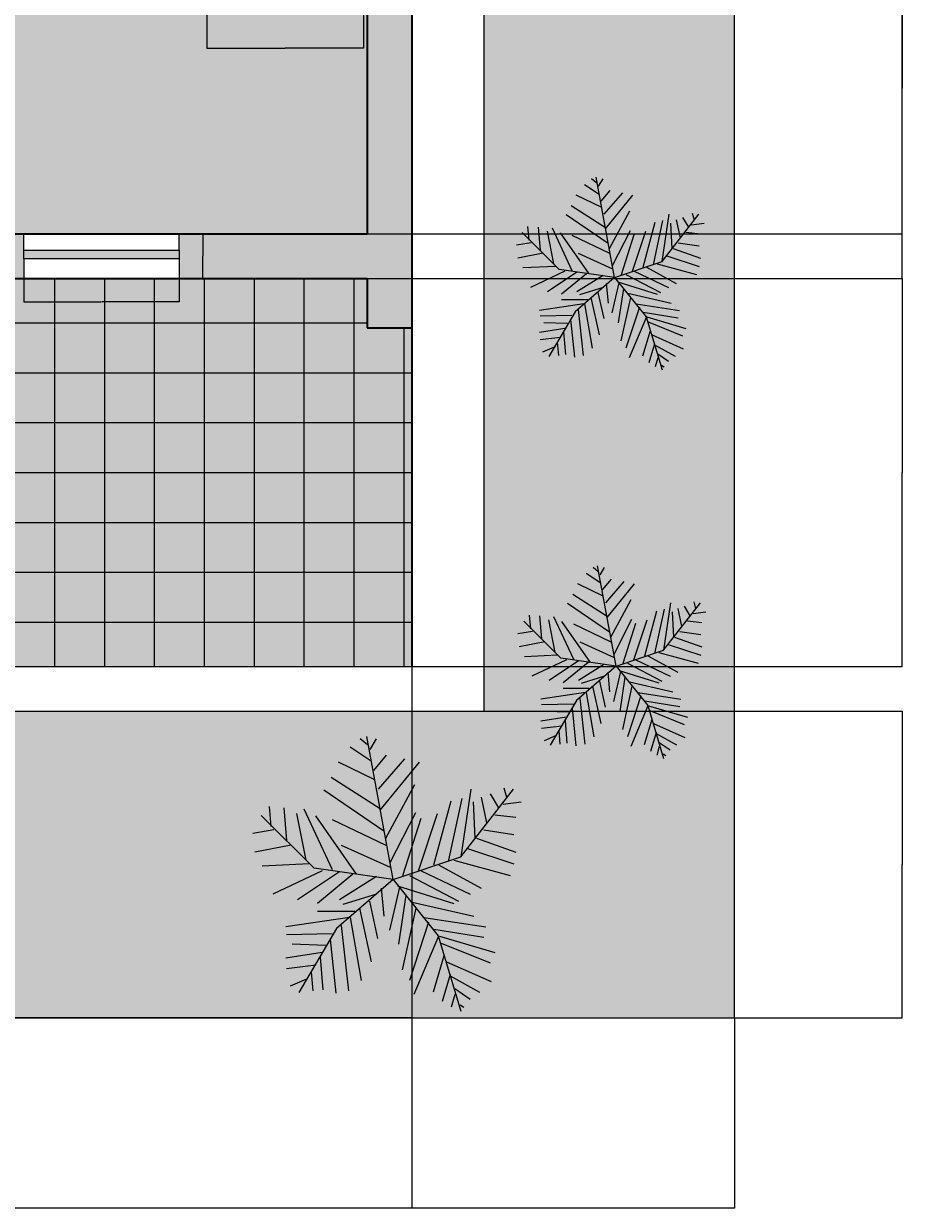
# Model space of a CAD drawing. Units: millimetres. Extents: x -229 to 16545, y -10488 to 4272.
# Tile 8 of 29: x 12015 to 16545, y -10230 to -4126. Entities that reach past the tile are written whole.
import ezdxf

# ---------------------------------------------------------------- set-up
doc = ezdxf.new("R2010")
doc.units = ezdxf.units.MM
for name, color, linetype, lineweight in [('A-ANNO-DIMS', 2, 'Continuous', 18), ('A-GLAZ', 4, 'Continuous', 18), ('A-WALL', 7, 'Continuous', 35), ('L-PLNT-BEDS', 82, 'Continuous', 18), ('L-PLNT-TREE', 80, 'Continuous', 18), ('L-PVMT', 7, 'Continuous', 18), ('L-PVMT-JNTS', 8, 'Continuous', 13)]:
    doc.layers.add(name, color=color, linetype=linetype, lineweight=lineweight)
for name, color, linetype, lineweight, true_color in [('A-FLOR-PATT', 254, 'Continuous', 13, 0xfeeab9), ('A-WALL-PATT', 18, 'Continuous', 13, 0x000000), ('L-PLNT-PATT', 116, 'Continuous', 13, 0x136734), ('L-PVMT-PATT', 252, 'Continuous', 13, 0x939598)]:
    doc.layers.add(name, color=color, linetype=linetype, lineweight=lineweight, true_color=true_color)
doc.styles.get("Standard").update_dxf_attribs({"font": 'arial.ttf'})
doc.dimstyles.get("Standard").update_dxf_attribs({"dimtxt": 0.18, "dimasz": 0.18, "dimexe": 0.18, "dimexo": 0.0625, "dimgap": 0.09, "dimtad": 0, "dimtih": 1, "dimtoh": 1, "dimdec": 4, "dimzin": 0, "dimdsep": 46, "dimtxsty": 'Standard', "dimcen": 0.09, "dimadec": 0, "dimazin": 0, "dimtfac": 1, "dimtdec": 4, "dimtofl": 0, "dimtmove": 0, "dimatfit": 3, "dimfxl": 1, "dimtolj": 1, "dimtzin": 0, "dimarcsym": 0})

# ---------------------------------------------------------------- blocks, each defined once
blk = doc.blocks.new('*U18')
for p, q in [((0, 0), (-10.5, 57)), ((-8.737, 47.138), (-17.069, 52.711)), ((-10.186, 53.64), (-13.084, 55.962)), ((-9.099, 51.782), (-6.563, 55.962)), ((-7.65, 43.423), (-2.578, 49.46)), ((-5.839, 35.992), (4.667, 48.067)), ((-7.288, 39.707), (-21.778, 46.673)), ((-5.114, 27.632), (10.463, 46.673)), ((-5.114, 28.097), (-24.676, 40.636)), ((-2.941, 16.486), (8.652, 37.85)), ((-3.665, 19.273), (-27.574, 35.527)), ((27, 9), (48, 36)), ((27.127, 9.056), (31.112, 35.992)), ((38.719, 34.134), (41.979, 28.561)), ((44.153, 36.456), (45.239, 32.741)), ((-48.585, 21.131), (-49.309, 29.026)), ((-43.513, 28.561), (-42.427, 15.558)), ((16.259, 5.805), (23.142, 31.348)), ((22.055, 7.198), (27.489, 32.277)), ((31.836, 30.883), (32.561, 16.486)), ((35.096, 32.741), (37.27, 22.524)), ((43.791, 29.954), (51.036, 30.883)), ((-31.5, 4.5), (-52.5, 25.5)), ((-38.442, 26.239), (-34.819, 7.663)), ((-35.544, 28.097), (-24.314, 3.947)), ((-14.533, 2.09), (-30.834, 25.31)), ((-24.314, 23.917), (-2.941, 13.7)), ((-1.129, 6.734), (9.014, 26.704)), ((3.942, 1.625), (11.187, 24.381)), ((10.101, 3.483), (17.708, 26.239)), ((40.53, 25.775), (48.862, 24.846)), ((-47.498, 19.737), (-55.83, 18.344)), ((36.183, 19.737), (48.137, 17.88)), ((33.285, 16.486), (48.862, 10.913)), ((-40.615, 13.7), (-55.105, 10.913)), ((-20.691, 13.7), (-1.129, 4.876)), ((29.662, 12.307), (48.137, 6.269)), ((-33.37, 6.269), (-52.207, 5.34)), ((0, 0), (27, 9)), ((18.07, 5.805), (35.096, -3.483)), ((24.229, 7.663), (46.688, 1.625)), ((-28.299, 3.483), (-47.86, -5.805)), ((-21.416, 3.018), (-38.079, -8.128)), ((0, 0), (-31.5, 4.5)), ((-15.982, 2.09), (-30.11, -9.521)), ((0, 0), (-22.5, -19.5)), ((-6.563, 1.161), (-21.416, -8.128)), ((0, 0), (18, -22.5)), ((6.478, 1.625), (26.04, -8.592)), ((11.187, 3.483), (30.749, -5.805)), ((-4.752, -3.483), (-3.665, -14.629)), ((2.493, -3.019), (-1.491, -20.202)), ((1.769, -2.555), (24.229, -9.521)), ((-6.563, -5.805), (-19.967, -9.985)), ((-9.461, -8.592), (-6.201, -23.453)), ((5.029, -6.27), (2.131, -25.775)), ((7.565, -9.056), (32.198, -14.629)), ((-15.257, -12.772), (-30.11, -12.772)), ((-13.446, -11.378), (-8.737, -32.741)), ((9.014, -11.378), (3.58, -35.992)), ((-17.431, -15.094), (-42.789, -18.809)), ((-20.691, -18.345), (-17.793, -44.352)), ((-17.069, -15.094), (-12.721, -40.172)), ((14.085, -16.951), (6.478, -40.172)), ((12.274, -15.094), (36.907, -18.809)), ((-24.314, -21.596), (-42.427, -22.06)), ((-22.5, -19.5), (-37.5, -45)), ((18.07, -22.524), (8.289, -45.745)), ((16.259, -19.738), (36.183, -22.989)), ((18, -22.5), (27, -52.5)), ((18.433, -22.524), (40.53, -29.026)), ((-26.849, -26.24), (-40.253, -25.775)), ((-25.038, -23.918), (-22.865, -45.281)), ((19.157, -25.311), (38.719, -33.206)), ((-28.299, -29.026), (-42.789, -31.348)), ((-29.023, -30.884), (-27.936, -43.887)), ((20.244, -30.419), (15.897, -44.816)), ((21.331, -32.741), (39.081, -40.636)), ((-30.834, -34.135), (-42.427, -35.528)), ((-32.646, -36.921), (-31.921, -44.352)), ((-34.457, -39.708), (-40.978, -42.494)), ((22.78, -37.85), (19.519, -48.532)), ((22.78, -38.314), (34.372, -44.816)), ((24.591, -45.745), (23.142, -50.854)), ((24.591, -43.423), (30.749, -47.603)), ((26.764, -49.925), (28.213, -50.854))]:
    blk.add_line(p, q)
blk = doc.blocks.new('WIN-802')
at = {"transparency": 33554687}
for p, q in [((0, 145), (0, 230)), ((802.3, 145), (802.3, 230)), ((0, 100.7), (0, 0)), ((802.3, 100.7), (802.3, 0))]:
    blk.add_line(p, q, dxfattribs=at)
blk.add_lwpolyline([(0, 145), (802.3, 145), (802.3, 100.7), (0, 100.7)], close=True, dxfattribs=at)
blk = doc.blocks.new('*D25')
at = {"layer": 'A-ANNO-DIMS', "color": 0, "lineweight": -2, "transparency": 16777216}
for p, q in [((12015.2, -5438.3), (12015.2, -5558.8)), ((12817.5, -5438.3), (12817.5, -5558.8)), ((12015.3, -5558.6), (12415.2, -5558.6)), ((12817.3, -5558.6), (12417.5, -5558.6))]:
    blk.add_line(p, q, dxfattribs=at)
at = {"layer": 'A-ANNO-DIMS', "color": 0, "transparency": 16777216}
for points in [[(12015.3, -5558.6), (12015.3, -5558.7), (12015.2, -5558.6)], [(12817.3, -5558.6), (12817.3, -5558.7), (12817.5, -5558.6)]]:
    blk.add_solid(points, dxfattribs=at)
at = {"layer": 'Defpoints', "color": 0, "transparency": 16777216}
for p in [(12015.2, -5438.3), (12817.5, -5438.3), (12817.5, -5558.6)]:
    blk.add_point(p, dxfattribs=at)
at = {"layer": 'A-ANNO-DIMS', "color": 0, "transparency": 16777216, "insert": (12416.3, -5558.6), "char_height": 0.18, "attachment_point": 5}
blk.add_mtext('\\A1;WINDOW 802 TYP.', dxfattribs=at)
blk = doc.blocks.new('*D26')
at = {"layer": 'A-ANNO-DIMS', "color": 0, "lineweight": -2, "transparency": 16777216}
for p, q in [((12817.6, -5208.3), (12938, -5208.3)), ((12937.9, -5208.5), (12937.9, -5323.1)), ((12937.9, -5438.1), (12937.9, -5323.5)), ((12817.6, -5438.3), (12938, -5438.3))]:
    blk.add_line(p, q, dxfattribs=at)
at = {"layer": 'A-ANNO-DIMS', "color": 0, "transparency": 16777216}
for points in [[(12937.8, -5208.5), (12937.9, -5208.5), (12937.9, -5208.3)], [(12937.8, -5438.1), (12937.9, -5438.1), (12937.9, -5438.3)]]:
    blk.add_solid(points, dxfattribs=at)
at = {"layer": 'Defpoints', "color": 0, "transparency": 16777216}
for p in [(12817.5, -5208.3), (12937.9, -5208.3), (12817.5, -5438.3)]:
    blk.add_point(p, dxfattribs=at)
at = {"layer": 'A-ANNO-DIMS', "color": 0, "transparency": 16777216, "insert": (12937.9, -5323.3), "char_height": 0.18, "attachment_point": 5}
blk.add_mtext('\\A1;230 TYP.', dxfattribs=at)
blk = doc.blocks.new('*D38')
at = {"layer": 'A-ANNO-DIMS', "color": 0, "lineweight": -2, "transparency": 16777216}
for p, q in [((12959.6, -3974.4), (12959.6, -4251.9)), ((13766.8, -3974.4), (13766.8, -4251.9)), ((12959.8, -4251.7), (13362.9, -4251.7)), ((13766.6, -4251.7), (13363.5, -4251.7))]:
    blk.add_line(p, q, dxfattribs=at)
at = {"layer": 'A-ANNO-DIMS', "color": 0, "transparency": 16777216}
for points in [[(12959.8, -4251.7), (12959.8, -4251.7), (12959.6, -4251.7)], [(13766.6, -4251.7), (13766.6, -4251.7), (13766.8, -4251.7)]]:
    blk.add_solid(points, dxfattribs=at)
at = {"layer": 'Defpoints', "color": 0, "transparency": 16777216}
for p in [(12959.6, -3974.3), (13766.8, -3974.3), (13766.8, -4251.7)]:
    blk.add_point(p, dxfattribs=at)
at = {"layer": 'A-ANNO-DIMS', "color": 0, "transparency": 16777216, "insert": (13363.2, -4251.7), "char_height": 0.18, "attachment_point": 5}
blk.add_mtext('\\A1;807', dxfattribs=at)
blk = doc.blocks.new('*D47')
at = {"layer": 'A-ANNO-DIMS', "color": 0, "lineweight": -2, "transparency": 16777216}
for p, q in [((912.1, -9248.3), (912.1, -10230.2)), ((15679.6, -9248.3), (15679.6, -10230.2)), ((912.2, -10230), (8295.4, -10230)), ((15679.4, -10230), (8296.3, -10230))]:
    blk.add_line(p, q, dxfattribs=at)
at = {"layer": 'A-ANNO-DIMS', "color": 0, "transparency": 16777216}
for points in [[(912.2, -10230), (912.2, -10230.1), (912.1, -10230)], [(15679.4, -10230), (15679.4, -10230.1), (15679.6, -10230)]]:
    blk.add_solid(points, dxfattribs=at)
at = {"layer": 'Defpoints', "color": 0, "transparency": 16777216}
for p in [(912.1, -9248.3), (15679.6, -9248.3), (15679.6, -10230)]:
    blk.add_point(p, dxfattribs=at)
at = {"layer": 'A-ANNO-DIMS', "color": 0, "transparency": 16777216, "insert": (8295.8, -10230), "char_height": 0.18, "attachment_point": 5}
blk.add_mtext('\\A1;14768', dxfattribs=at)
blk = doc.blocks.new('*D48')
at = {"layer": 'A-ANNO-DIMS', "color": 0, "lineweight": -2, "transparency": 16777216}
for p, q in [((14016, 2251.7), (16544.5, 2251.7)), ((16544.3, 2251.5), (16544.3, -1593.1)), ((16544.3, -5438.1), (16544.3, -1593.5)), ((13786, -5438.3), (16544.5, -5438.3))]:
    blk.add_line(p, q, dxfattribs=at)
at = {"layer": 'A-ANNO-DIMS', "color": 0, "transparency": 16777216}
for points in [[(16544.3, 2251.5), (16544.4, 2251.5), (16544.3, 2251.7)], [(16544.3, -5438.1), (16544.4, -5438.1), (16544.3, -5438.3)]]:
    blk.add_solid(points, dxfattribs=at)
at = {"layer": 'Defpoints', "color": 0, "transparency": 16777216}
for p in [(14015.9, 2251.7), (13785.9, -5438.3), (16544.3, -5438.3)]:
    blk.add_point(p, dxfattribs=at)
at = {"layer": 'A-ANNO-DIMS', "color": 0, "transparency": 16777216, "insert": (16544.3, -1593.3), "char_height": 0.18, "attachment_point": 5}
blk.add_mtext('\\A1;7690', dxfattribs=at)
blk = doc.blocks.new('*D57')
at = {"layer": 'A-ANNO-DIMS', "color": 0, "lineweight": -2, "transparency": 16777216}
for p, q in [((13786, -1208.3), (16544.5, -1208.3)), ((16544.3, -1208.5), (16544.3, -3208.1)), ((16544.3, -5208.1), (16544.3, -3208.5)), ((13786, -5208.3), (16544.5, -5208.3))]:
    blk.add_line(p, q, dxfattribs=at)
at = {"layer": 'A-ANNO-DIMS', "color": 0, "transparency": 16777216}
for points in [[(16544.3, -1208.5), (16544.4, -1208.5), (16544.3, -1208.3)], [(16544.3, -5208.1), (16544.4, -5208.1), (16544.3, -5208.3)]]:
    blk.add_solid(points, dxfattribs=at)
at = {"layer": 'Defpoints', "color": 0, "transparency": 16777216}
for p in [(13785.9, -1208.3), (13785.9, -5208.3), (16544.3, -5208.3)]:
    blk.add_point(p, dxfattribs=at)
at = {"layer": 'A-ANNO-DIMS', "color": 0, "transparency": 16777216, "insert": (16544.3, -3208.3), "char_height": 0.18, "attachment_point": 5}
blk.add_mtext('\\A1;4000', dxfattribs=at)
blk = doc.blocks.new('*D60')
at = {"layer": 'A-ANNO-DIMS', "color": 0, "lineweight": -2, "transparency": 16777216}
for p, q in [((8205.9, -7438.3), (8205.9, -10230.2)), ((14015.9, -7438.3), (14015.9, -10230.2)), ((8206.1, -10230), (11110.6, -10230)), ((14015.8, -10230), (11111.3, -10230))]:
    blk.add_line(p, q, dxfattribs=at)
at = {"layer": 'A-ANNO-DIMS', "color": 0, "transparency": 16777216}
for points in [[(8206.1, -10230), (8206.1, -10230.1), (8205.9, -10230)], [(14015.8, -10230), (14015.8, -10230.1), (14015.9, -10230)]]:
    blk.add_solid(points, dxfattribs=at)
at = {"layer": 'Defpoints', "color": 0, "transparency": 16777216}
for p in [(8205.9, -7438.3), (14015.9, -7438.3), (14015.9, -10230)]:
    blk.add_point(p, dxfattribs=at)
at = {"layer": 'A-ANNO-DIMS', "color": 0, "transparency": 16777216, "insert": (11110.9, -10230), "char_height": 0.18, "attachment_point": 5}
blk.add_mtext('\\A1;5810', dxfattribs=at)
blk = doc.blocks.new('*D61')
at = {"layer": 'A-ANNO-DIMS', "color": 0, "lineweight": -2, "transparency": 16777216}
for p, q in [((8206, -5438.3), (16544.5, -5438.3)), ((16544.3, -5438.5), (16544.3, -6438.1)), ((16544.3, -7438.1), (16544.3, -6438.5)), ((8206, -7438.3), (16544.5, -7438.3))]:
    blk.add_line(p, q, dxfattribs=at)
at = {"layer": 'A-ANNO-DIMS', "color": 0, "transparency": 16777216}
for points in [[(16544.3, -5438.5), (16544.4, -5438.5), (16544.3, -5438.3)], [(16544.3, -7438.1), (16544.4, -7438.1), (16544.3, -7438.3)]]:
    blk.add_solid(points, dxfattribs=at)
at = {"layer": 'Defpoints', "color": 0, "transparency": 16777216}
for p in [(8205.9, -5438.3), (16544.3, -5438.3), (8205.9, -7438.3)]:
    blk.add_point(p, dxfattribs=at)
at = {"layer": 'A-ANNO-DIMS', "color": 0, "transparency": 16777216, "insert": (16544.3, -6438.3), "char_height": 0.18, "attachment_point": 5}
blk.add_mtext('\\A1;2000', dxfattribs=at)
blk = doc.blocks.new('*D79')
at = {"layer": 'A-ANNO-DIMS', "color": 0, "lineweight": -2, "transparency": 16777216}
for p, q in [((8206, -7668.3), (16544.5, -7668.3)), ((16544.3, -7668.5), (16544.3, -8458.1)), ((16544.3, -9248.1), (16544.3, -8458.5)), ((8209.2, -9248.3), (16544.5, -9248.3))]:
    blk.add_line(p, q, dxfattribs=at)
at = {"layer": 'A-ANNO-DIMS', "color": 0, "transparency": 16777216}
for points in [[(16544.3, -7668.5), (16544.4, -7668.5), (16544.3, -7668.3)], [(16544.3, -9248.1), (16544.4, -9248.1), (16544.3, -9248.3)]]:
    blk.add_solid(points, dxfattribs=at)
at = {"layer": 'Defpoints', "color": 0, "transparency": 16777216}
for p in [(8205.9, -7668.3), (8209.2, -9248.3), (16544.3, -9248.3)]:
    blk.add_point(p, dxfattribs=at)
at = {"layer": 'A-ANNO-DIMS', "color": 0, "transparency": 16777216, "insert": (16544.3, -8458.3), "char_height": 0.18, "attachment_point": 5}
blk.add_mtext('\\A1;1580', dxfattribs=at)
blk = doc.blocks.new('*D87')
at = {"layer": 'A-ANNO-DIMS', "color": 0, "lineweight": -2, "transparency": 16777216}
for p, q in [((13786, -3709.5), (16544.5, -3709.5)), ((16544.3, -3709.7), (16544.3, -4458.7)), ((16544.3, -5208.1), (16544.3, -4459.1)), ((13786, -5208.3), (16544.5, -5208.3))]:
    blk.add_line(p, q, dxfattribs=at)
at = {"layer": 'A-ANNO-DIMS', "color": 0, "transparency": 16777216}
for points in [[(16544.3, -3709.7), (16544.4, -3709.7), (16544.3, -3709.5)], [(16544.3, -5208.1), (16544.4, -5208.1), (16544.3, -5208.3)]]:
    blk.add_solid(points, dxfattribs=at)
at = {"layer": 'Defpoints', "color": 0, "transparency": 16777216}
for p in [(13785.9, -3709.5), (16544.3, -3709.5), (13785.9, -5208.3)]:
    blk.add_point(p, dxfattribs=at)
at = {"layer": 'A-ANNO-DIMS', "color": 0, "transparency": 16777216, "insert": (16544.3, -4458.9), "char_height": 0.18, "attachment_point": 5}
blk.add_mtext('\\A1;1498.7', dxfattribs=at)

msp = doc.modelspace()

# ---------------------------------------------------------------- hatches: boundary and pattern name
at = {"layer": 'A-FLOR-PATT', "transparency": 33554592}
h = msp.add_hatch(color=256, dxfattribs=at)
h.dxf.hatch_style = 1
h.paths.add_polyline_path([(7975.933, -5325.772), (7943.121, -5325.772), (7943.121, -4576.49, 0.40145271), (7225.933, -5325.772, 0.40145271), (6508.746, -4576.49), (6508.746, -5325.772), (6475.933, -5325.772), (6475.933, -5438.272), (5975.933, -5438.272), (5975.933, -7267.724), (5975.933, -7438.272), (6478.619, -7438.272), (6463.448, -7355.919), (6464.88, -7356.837), (6463.849, -7358.097), (6478.619, -7438.272), (6610.327, -7438.272), (6632.656, -7409.564), (6632.525, -7406.967), (6634.208, -7407.569), (6619.273, -7426.77), (6654.466, -7438.272), (7610.517, -7438.272), (7607.41, -7421.409), (7608.842, -7422.327), (7607.812, -7423.587), (7610.517, -7438.272), (7975.933, -7438.272)])
h.paths.add_polyline_path([(13785.933, -1208.272), (9555.933, -1208.272), (9555.933, -961.785), (9705.933, -961.785), (9705.933, -918.035), (10704.976, -918.035, 0.40145271), (9705.933, 38.215), (9555.933, 38.215), (9555.933, 2021.728), (5975.933, 2021.728), (5975.933, 755.492), (5745.933, 755.492), (5745.933, 1427.266), (2918.813, 1427.266), (2918.813, -492.942), (5013.319, -492.942), (5013.319, -978.272), (5745.933, -978.272), (5745.933, -397.513), (5975.933, -397.513), (5975.933, -1208.272), (4560.933, -1208.272), (4560.933, -1265.772), (4448.433, -1265.772), (4448.433, -1298.585), (4445.933, -1298.585), (3699.151, -1298.585, 0.40145271), (4448.433, -2015.772), (4560.933, -2015.772), (4560.933, -2384.177), (5745.933, -2384.177), (5799.402, -2384.177), (5799.402, -4518.272), (5975.933, -4518.272), (5975.933, -5208.272), (6475.933, -5208.272), (6475.933, -4575.772), (6508.746, -4575.772), (6508.746, -4576.49, -0.35647263), (7216.672, -5208.272), (7235.194, -5208.272, -0.35647263), (7943.121, -4576.49), (7943.121, -4575.772), (7975.933, -4575.772), (7975.933, -5208.272), (11176.247, -5208.272), (11159.44, -5191.465), (10520.768, -5191.465), (10520.768, -4888.936), (10571.19, -4888.936), (10571.19, -4872.129), (10772.876, -4872.129), (10772.876, -4888.936), (10789.683, -4888.936), (10789.683, -4872.129), (10991.368, -4872.129), (10991.368, -4888.936), (11041.79, -4888.936), (11041.79, -4872.129), (11058.597, -4872.129, -0.09090909), (11428.354, -4872.129), (11445.162, -4872.129), (11445.162, -4888.936), (11529.197, -4888.936), (11529.197, -5191.465), (11327.512, -5191.465), (11310.704, -5208.272), (13785.933, -5208.272)])
h.paths.add_polyline_path([(11047.216, -1630.944, -1), (11402.816, -1630.944, -1)], flags=16)
h.paths.add_polyline_path([(11148.816, -1630.944), (11225.016, -1554.744), (11301.216, -1630.944), (11225.016, -1707.144)], flags=0)
h.paths.add_polyline_path([(11199.616, -1630.944, -1), (11250.416, -1630.944, -1)], flags=0)
h.paths.add_polyline_path([(11588.751, -2096.259), (11588.751, -1543.254, -0.26666697), (12864.918, -1543.254), (12864.918, -2096.259), (12737.302, -2096.259), (12737.302, -2063.121), (11716.368, -2063.121), (11716.368, -2096.259)], flags=16)
h.paths.add_polyline_path([(12012.696, -2489.42), (12600.997, -2489.42), (12600.997, -3666.022), (12012.696, -3666.022)], flags=16)
h.paths.add_polyline_path([(12176.41, -3599.403), (12174.938, -3609.076), (12173.789, -3618.819), (12173.09, -3628.559), (12172.973, -3638.221), (12173.89, -3652.852), (12175.008, -3657.025), (12172.909, -3643.473), (12173.142, -3624.297), (12175.386, -3605.273)], flags=0)
h.paths.add_polyline_path([(8026.289, -286.944), (7737.703, -287.19), (7734.87, -269.156), (8029.092, -268.905)], flags=16)
h.paths.add_polyline_path([(7733.453, -260.139), (7710.784, -115.865), (7557.191, -115.996), (7556.999, 109.744), (7412.687, 132.166), (7412.433, 429.206), (7556.707, 451.876), (7556.568, 614.769), (7412.256, 637.19), (7412.003, 934.231), (7556.276, 956.9), (7556.084, 1182.639), (7709.677, 1182.77), (7732.099, 1327.082), (8029.14, 1327.335), (8051.808, 1183.062), (8205.401, 1183.192), (8205.594, 957.454), (8349.906, 935.031), (8350.159, 637.99), (8205.885, 615.322), (8206.024, 452.43), (8350.336, 430.006), (8350.59, 132.965), (8206.316, 110.298), (8206.509, -115.442), (8052.916, -115.573), (8030.493, -259.885)], flags=16)
h.paths.add_polyline_path([(12261.416, -3475.554), (12262.632, -3486.776), (12264.032, -3497.007), (12265.554, -3506.365), (12267.136, -3514.968), (12268.719, -3522.935), (12271.304, -3535.59), (12273.606, -3548.078), (12275.271, -3561.064), (12275.93, -3574.938), (12275.325, -3590.3), (12273.425, -3607.964), (12270.795, -3625.658), (12268.066, -3641.063), (12266.318, -3649.679), (12265.456, -3653.626), (12263.984, -3659.846), (12264.032, -3659.566), (12264.342, -3658.241), (12264.807, -3656.37), (12265.456, -3653.626), (12266.318, -3649.679), (12267.409, -3644.302), (12268.668, -3637.664), (12270.019, -3630.037), (12271.384, -3621.695), (12272.69, -3612.908), (12273.857, -3603.948), (12274.81, -3595.088), (12275.47, -3586.601), (12275.782, -3578.689), (12275.757, -3571.292), (12275.423, -3564.275), (12274.816, -3557.512), (12273.964, -3550.872), (12272.896, -3544.224), (12271.645, -3537.439), (12270.24, -3530.385), (12267.543, -3517.181), (12264.612, -3501.247), (12261.849, -3481.059)], flags=0)
h.paths.add_polyline_path([(12332.136, -3408.03), (12333.483, -3416.79), (12335.077, -3424.54), (12336.915, -3431.355), (12338.991, -3437.32), (12341.266, -3442.55), (12343.694, -3447.166), (12346.229, -3451.292), (12348.826, -3455.051), (12351.438, -3458.563), (12357.476, -3466.491), (12363.61, -3476.575), (12368.309, -3489.762), (12369.929, -3503.427), (12369.842, -3516.511), (12368.43, -3530.867), (12365.816, -3545.835), (12362.382, -3559.786), (12360.968, -3564.487), (12363.063, -3557.021), (12364.898, -3549.566), (12366.473, -3542.077), (12367.773, -3534.631), (12368.781, -3527.301), (12369.483, -3520.162), (12369.863, -3513.291), (12369.906, -3506.759), (12369.599, -3500.643), (12368.93, -3494.999), (12367.924, -3489.796), (12366.61, -3484.994), (12365.024, -3480.542), (12363.19, -3476.399), (12361.141, -3472.516), (12358.909, -3468.847), (12356.525, -3465.347), (12354.02, -3461.954), (12351.438, -3458.563), (12345.462, -3450.529), (12339.923, -3439.996), (12335.85, -3428.296), (12332.68, -3412.888)], flags=0)
h.paths.add_polyline_path([(12385.287, -3334.612), (12384.977, -3342.409), (12385.02, -3349.196), (12385.4, -3355.066), (12386.104, -3360.105), (12387.112, -3364.41), (12388.412, -3368.071), (12389.987, -3371.181), (12391.823, -3373.832), (12393.919, -3376.097), (12396.337, -3377.978), (12399.153, -3379.462), (12402.445, -3380.531), (12406.289, -3381.172), (12410.758, -3381.371), (12415.935, -3381.106), (12421.893, -3380.368), (12428.658, -3379.159), (12436.069, -3377.55), (12443.907, -3375.635), (12451.961, -3373.505), (12460.015, -3371.254), (12467.853, -3368.971), (12475.263, -3366.749), (12482.029, -3364.68), (12491.877, -3361.657), (12497.701, -3360.107), (12501.639, -3359.288), (12510.135, -3358.326), (12519.662, -3365.412), (12524.243, -3378.911), (12523.764, -3390.7), (12520.746, -3401.577), (12514.248, -3415.634), (12511.518, -3420.418), (12515.856, -3412.154), (12519.153, -3405.024), (12521.516, -3398.804), (12523.049, -3393.276), (12523.865, -3388.212), (12524.059, -3383.441), (12523.7, -3378.958), (12522.853, -3374.815), (12521.576, -3371.054), (12519.931, -3367.722), (12517.982, -3364.865), (12515.786, -3362.529), (12513.405, -3360.758), (12510.877, -3359.588), (12508.136, -3358.982), (12505.086, -3358.897), (12501.639, -3359.288), (12497.701, -3360.107), (12493.183, -3361.309), (12487.988, -3362.851), (12476.403, -3366.408), (12463.335, -3370.326), (12447.372, -3374.788), (12431.759, -3378.604), (12418.504, -3380.974), (12405.811, -3381.624), (12394.725, -3378.025), (12388.039, -3368.367), (12385.583, -3357.877), (12384.826, -3346.204), (12385.428, -3331.059), (12385.953, -3325.719)], flags=0)
h.paths.add_polyline_path([(7880.016, 1173.969), (7880.373, 1175.495), (7880.433, 1175.851), (7879.484, 1171.818)], flags=0)
h.paths.add_polyline_path([(7802.33, 874.962), (7800.771, 885.032), (7798.932, 893.941), (7796.811, 901.774), (7794.419, 908.63), (7791.798, 914.639), (7789.002, 919.945), (7786.083, 924.686), (7783.093, 929.005), (7780.087, 933.043), (7774.996, 939.717), (7768.406, 949.37), (7762.174, 963.427), (7759.342, 978.002), (7758.629, 991.888), (7759.492, 1007.928), (7761.801, 1025.496), (7765.392, 1044.035), (7766.625, 1049.048), (7764.522, 1039.543), (7762.719, 1030.232), (7761.232, 1021.168), (7760.08, 1012.405), (7759.28, 1003.994), (7758.849, 995.988), (7758.806, 988.44), (7759.167, 981.404), (7759.942, 974.914), (7761.104, 968.936), (7762.617, 963.414), (7764.448, 958.299), (7766.559, 953.535), (7768.918, 949.073), (7771.487, 944.856), (7774.232, 940.835), (7777.115, 936.938), (7782.377, 930.041), (7787.845, 922.139), (7793.348, 911.698), (7798.042, 898.247), (7801.702, 880.527)], flags=0)
h.paths.add_polyline_path([(12519.068, -3228.534), (12519.615, -3236.235), (12520.529, -3242.343), (12521.78, -3247.103), (12523.337, -3250.758), (12525.171, -3253.556), (12527.248, -3255.709), (12529.522, -3257.296), (12531.95, -3258.361), (12534.486, -3258.949), (12537.082, -3259.11), (12539.694, -3258.888), (12542.277, -3258.329), (12544.781, -3257.478), (12547.173, -3256.388), (12549.46, -3255.129), (12550.455, -3254.517), (12555.825, -3251.109), (12557.835, -3249.942), (12565.181, -3246.404), (12574.565, -3253.032), (12576.931, -3265.022), (12576.627, -3277.425), (12575.416, -3290.819), (12574.851, -3295.392), (12575.708, -3287.593), (12576.322, -3280.806), (12576.688, -3274.939), (12576.812, -3269.899), (12576.688, -3265.593), (12576.322, -3261.932), (12575.708, -3258.822), (12574.851, -3256.172), (12573.753, -3253.905), (12572.439, -3252.005), (12570.943, -3250.474), (12569.293, -3249.309), (12567.523, -3248.513), (12565.658, -3248.083), (12563.732, -3248.022), (12561.777, -3248.328), (12559.814, -3248.989), (12557.835, -3249.942), (12555.825, -3251.109), (12553.77, -3252.413), (12551.652, -3253.78), (12549.46, -3255.129), (12543.167, -3258.594), (12532.661, -3259.485), (12524.685, -3253.923), (12520.949, -3245.152), (12519.138, -3233.042)], flags=0)
h.paths.add_polyline_path([(7741.293, 790.501), (7741.641, 799.467), (7741.584, 807.269), (7741.141, 814.015), (7740.329, 819.809), (7739.165, 824.757), (7737.667, 828.966), (7735.853, 832.541), (7733.74, 835.586), (7731.348, 838.188), (7728.71, 840.348), (7725.861, 842.052), (7722.836, 843.28), (7719.671, 844.015), (7716.4, 844.237), (7713.06, 843.932), (7709.684, 843.081), (7706.304, 841.686), (7702.923, 839.834), (7699.543, 837.629), (7696.164, 835.178), (7692.784, 832.585), (7684.718, 826.315), (7675.609, 820.63), (7664.001, 817.274), (7654.105, 821.884), (7647.171, 832.02), (7644.191, 846.522), (7646.321, 860.288), (7647.49, 864.223), (7645.946, 857.865), (7645.046, 852.044), (7644.827, 846.557), (7645.243, 841.404), (7646.221, 836.642), (7647.693, 832.318), (7649.587, 828.489), (7651.832, 825.206), (7654.359, 822.523), (7657.097, 820.49), (7659.984, 819.145), (7662.993, 818.452), (7666.108, 818.357), (7669.311, 818.809), (7672.583, 819.755), (7675.908, 821.139), (7679.268, 822.913), (7682.645, 825.021), (7686.025, 827.401), (7689.404, 829.958), (7692.784, 832.585), (7700.505, 838.509), (7709.871, 843.64), (7721.436, 844.698), (7733.277, 837.617), (7739.571, 825.214), (7741.557, 811.049), (7741.669, 795.575)], flags=0)
h.paths.add_polyline_path([(8377.641, 137.216), (8359.607, 134.382), (8359.356, 428.605), (8377.395, 425.802)], flags=16)
h.paths.add_polyline_path([(7650.715, 668.465), (7650.08, 677.319), (7649.023, 684.34), (7647.579, 689.811), (7645.785, 694.012), (7643.675, 697.228), (7641.286, 699.7), (7638.669, 701.521), (7635.876, 702.744), (7632.96, 703.419), (7629.974, 703.601), (7626.971, 703.344), (7624.004, 702.697), (7621.125, 701.717), (7618.375, 700.462), (7615.749, 699.013), (7614.561, 698.279), (7608.435, 694.382), (7606.125, 693.04), (7598.981, 689.594), (7589.669, 693.773), (7585.26, 702.856), (7584.221, 713.11), (7584.49, 724.584), (7585.863, 739.937), (7586.518, 745.277), (7585.539, 736.31), (7584.841, 728.507), (7584.424, 721.761), (7584.288, 715.966), (7584.433, 711.016), (7584.86, 706.807), (7585.567, 703.231), (7586.556, 700.186), (7587.821, 697.58), (7589.332, 695.397), (7591.053, 693.637), (7592.951, 692.3), (7594.989, 691.385), (7597.132, 690.895), (7599.346, 690.826), (7601.594, 691.18), (7603.851, 691.943), (7606.125, 693.04), (7608.435, 694.382), (7610.797, 695.885), (7613.229, 697.458), (7620.475, 701.929), (7632.001, 704.44), (7643.476, 699.417), (7648.536, 687.571), (7650.63, 673.661)], flags=0)
h.paths.add_polyline_path([(7385.628, 136.37), (7385.382, 424.956), (7403.416, 427.789), (7403.667, 133.567)], flags=16)
h.paths.add_polyline_path([(12993.884, -2257.186), (12959.588, -2257.186), (12959.588, -2125.099), (13531.966, -2125.099, -0.19047621), (13531.966, -3974.321), (12959.588, -3974.321), (12959.588, -3842.233), (12993.884, -3842.233)], flags=16)
h.paths.add_polyline_path([(13413.486, -3313.884), (13413.486, -2785.535), (13562.885, -2785.535, -0.04962821), (13562.885, -3313.884)], flags=0)
h.paths.add_polyline_path([(8377.21, 642.241), (8359.176, 639.407), (8358.925, 933.629), (8376.964, 930.826)], flags=16)
h.paths.add_polyline_path([(13086.058, -1864.83), (13086.058, -1449.84), (13501.048, -1449.84), (13501.048, -1864.83)], flags=16)
h.paths.add_polyline_path([(13305.814, -1862.197), (13302.103, -1859.624), (13298.088, -1857.068), (13293.799, -1854.536), (13289.262, -1852.031), (13284.504, -1849.559), (13279.554, -1847.125), (13274.439, -1844.735), (13269.17, -1842.389), (13263.701, -1840.081), (13257.97, -1837.797), (13251.914, -1835.525), (13245.472, -1833.252), (13238.582, -1830.968), (13231.18, -1828.66), (13223.206, -1826.315), (13209.182, -1822.458), (13204.584, -1821.48), (13217.962, -1824.773), (13235.072, -1829.804), (13248.777, -1834.349), (13260.829, -1838.869), (13274.479, -1844.63), (13289.675, -1852.101), (13302.553, -1859.704)], flags=0)
h.paths.add_polyline_path([(13428.104, -1820.994), (13419.007, -1818.141), (13409.95, -1815.4), (13400.766, -1812.747), (13391.271, -1810.151), (13376.087, -1806.251), (13370.618, -1805.019), (13386.304, -1808.794), (13405.087, -1813.928), (13423.014, -1819.354)], flags=0)
h.paths.add_polyline_path([(7385.197, 641.395), (7384.951, 929.98), (7402.986, 932.814), (7403.236, 638.592)], flags=16)
h.paths.add_polyline_path([(13262.537, -1725.526), (13253.246, -1724.74), (13244.516, -1724.117), (13235.94, -1723.625), (13223.267, -1723.062), (13217.598, -1722.912), (13231.966, -1723.397), (13248.733, -1724.359), (13266.899, -1725.895), (13272.802, -1726.502)], flags=0)
h.paths.add_polyline_path([(13191.893, -1641.137), (13208.675, -1640.506), (13214.057, -1640.258), (13197.763, -1640.936)], flags=0)
h.paths.add_polyline_path([(13097.524, -1608.457), (13114.284, -1609.031), (13120.126, -1609.105), (13103.045, -1608.71)], flags=0)
h.paths.add_polyline_path([(13465.328, -1521.577), (13473.906, -1517.015), (13481.761, -1511.636), (13492.562, -1502.076), (13495.327, -1497.933), (13485.818, -1508.858), (13470.208, -1519.547)], flags=0)
h.paths.add_polyline_path([(13175.015, -1500.891), (13184.046, -1501.807), (13192.721, -1502.52), (13201.114, -1503.034), (13209.273, -1503.351), (13217.244, -1503.476), (13225.078, -1503.41), (13232.821, -1503.16), (13240.524, -1502.728), (13248.233, -1502.117), (13255.993, -1501.322), (13263.825, -1500.293), (13271.746, -1498.974), (13279.775, -1497.305), (13287.928, -1495.229), (13296.222, -1492.688), (13304.675, -1489.622), (13313.304, -1485.975), (13322.089, -1481.727), (13330.859, -1477.028), (13339.408, -1472.063), (13347.526, -1467.02), (13355.006, -1462.087), (13364.86, -1455.202), (13367.224, -1453.299), (13358.544, -1459.754), (13343.348, -1469.775), (13326.143, -1479.767), (13309.023, -1488.045), (13292.249, -1494.129), (13276.009, -1498.264), (13260.299, -1500.88), (13244.401, -1502.51), (13228.945, -1503.378), (13213.316, -1503.508), (13197.047, -1502.876), (13180.088, -1501.481)], flags=0)
h.paths.add_polyline_path([(7733.501, 1336.101), (7736.303, 1354.14), (8024.889, 1354.386), (8027.723, 1336.352)], flags=16)
at = {"layer": 'A-WALL-PATT'}
h = msp.add_hatch(color=256, dxfattribs=at)
h.dxf.hatch_style = 1
h.paths.add_polyline_path([(7294.425, 2163.983), (7294.425, 2251.728), (4412.722, 2251.728), (4412.722, 2166.741), (4412.722, 2122.457), (4412.722, 2021.728), (7294.425, 2021.728), (7294.425, 2119.698)])
h.paths.add_polyline_path([(11407.51, 2166.741), (11407.51, 2251.728), (8296.763, 2251.728), (8296.763, 2163.983), (8296.763, 2119.698), (8296.763, 2021.728), (11407.51, 2021.728), (11407.51, 2122.457)])
h.paths.add_polyline_path([(9785.933, 2021.728), (9555.933, 2021.728), (9555.933, 38.215), (9705.933, 38.215, -0.02002407), (9785.933, 35.01)])
h.paths.add_polyline_path([(14015.933, 2251.728), (12488.002, 2251.728), (12488.002, 2166.742), (12488.002, 2122.738), (12488.002, 2021.728), (13785.933, 2021.728), (13785.933, -2305.465), (13883.903, -2305.465), (13928.188, -2305.465), (14015.933, -2305.465)])
h.paths.add_polyline_path([(13785.933, -978.272), (9785.933, -978.272), (9785.933, -961.785), (9705.933, -961.785), (9555.933, -961.785), (9555.933, -1208.272), (13785.933, -1208.272)])
h.paths.add_polyline_path([(5975.933, 2021.728), (5745.933, 2021.728), (5745.933, 755.492), (5975.933, 755.492)])
h.paths.add_polyline_path([(2245.933, 2021.728), (3420.865, 2021.728), (3420.865, 2122.457), (3420.865, 2167.104), (3420.865, 2251.728), (2015.933, 2251.728), (2015.933, -3326.811), (2100.943, -3326.811), (2155.199, -3326.811), (2245.933, -3326.811)])
h.paths.add_polyline_path([(5975.933, -397.513), (5745.933, -397.513), (5745.933, -978.272), (2245.933, -978.272), (2245.933, -1208.272), (5975.933, -1208.272)])
h.paths.add_polyline_path([(12015.17, -5208.272), (7975.933, -5208.272), (7975.933, -5325.772), (7975.933, -5438.272), (7975.933, -5596.884), (8205.933, -5596.884), (8205.933, -5438.272), (12015.17, -5438.272), (12015.17, -5337.543), (12015.17, -5293.259)])
h.paths.add_polyline_path([(5975.933, -4518.272), (4567.83, -4518.272), (4567.83, -4603.259), (4567.83, -4647.543), (4567.83, -4748.272), (5745.933, -4748.272), (5745.933, -5438.272), (5975.933, -5438.272), (6475.933, -5438.272), (6475.933, -5325.772), (6475.933, -5208.272), (5975.933, -5208.272)])
h.paths.add_polyline_path([(3765.491, -4518.272), (2245.933, -4518.272), (2245.933, -4748.272), (3765.491, -4748.272), (3765.491, -4647.543), (3765.491, -4603.259)])
h = msp.add_hatch(color=256, dxfattribs=at)
h.dxf.hatch_style = 1
h.paths.add_polyline_path([(13883.903, -2305.465), (13928.188, -2305.465), (13928.188, -3709.532), (14015.933, -3709.532), (14015.933, -5692.852), (13785.933, -5692.852), (13785.933, -5438.272), (12817.508, -5438.272), (12817.508, -5337.543), (12015.17, -5337.543), (12015.17, -5293.259), (12817.508, -5293.259), (12817.508, -5208.272), (13785.933, -5208.272), (13785.933, -3709.532), (13883.903, -3709.532)])
at = {"layer": 'L-PLNT-PATT'}
h = msp.add_hatch(dxfattribs=at)
h.set_pattern_fill('GRASS', color=256, scale=2)
h.set_pattern_definition([(90, (-8141.222, -13125.504), (-35.921024, 35.921024), [9.525, -62.31705]), (45, (-8141.22, -13125.504), (-35.92102, 35.92102), [9.525, -41.275]), (135, (-8141.22, -13125.504), (-35.92102, -35.92102), [9.525, -41.275])])
h.paths.add_polyline_path([(15679.607, 2251.728), (14387.79, 2251.728), (14387.79, -7668.272), (8209.16, -7668.272), (8209.16, -9248.272), (14015.933, -9248.272), (15679.607, -9248.272)])
at = {"layer": 'L-PVMT-JNTS', "transparency": 33554541}
h = msp.add_hatch(dxfattribs=at)
h.set_pattern_fill('NET', color=256, scale=81)
h.set_pattern_definition([(0, (-8141.22, -13125.5), (0, 257.175), []), (90, (-8141.22, -13125.5), (-257.175, 2e-14), [])])
h.paths.add_polyline_path([(14015.933, -5692.852), (13785.933, -5692.852), (13785.933, -5438.272), (8205.933, -5438.272), (8205.933, -7438.272), (14015.933, -7438.272)])
at = {"layer": 'L-PVMT-PATT', "transparency": 33554541}
h = msp.add_hatch(color=256, dxfattribs=at)
h.dxf.hatch_style = 1
h.paths.add_polyline_path([(14015.933, -5692.852), (13785.933, -5692.852), (13785.933, -5438.272), (8205.933, -5438.272), (8205.933, -7438.272), (14015.933, -7438.272)])

# ---------------------------------------------------------------- linework, layer by layer
at = {"layer": 'A-WALL'}
for p, q in [((14015.933, 2251.728), (14015.933, -7438.272)), ((13785.933, 2021.728), (13785.933, -5208.272)), ((7943.121, -5208.272), (13785.933, -5208.272)), ((8205.933, -5438.272), (13785.933, -5438.272)), ((13785.933, -5438.272), (13785.933, -5692.852)), ((13785.933, -5692.852), (14015.933, -5692.852))]:
    msp.add_line(p, q, dxfattribs=at)
at = {"layer": 'L-PLNT-BEDS', "transparency": 33554572}
msp.add_line((14387.79, 2251.728), (14387.79, -7668.272), dxfattribs=at)
at = {"layer": 'L-PLNT-BEDS', "transparency": 33554554}
for p, q in [((15679.607, -9248.272), (15679.607, 2251.728)), ((14015.933, -9248.272), (15679.607, -9248.272))]:
    msp.add_line(p, q, dxfattribs=at)
at = {"layer": 'L-PLNT-BEDS'}
msp.add_line((8205.933, -7668.272), (14387.79, -7668.272), dxfattribs=at)
at = {"layer": 'L-PVMT'}
for p, q in [((8205.933, -7438.272), (14015.933, -7438.272)), ((14015.933, -9248.272), (2015.933, -9248.272))]:
    msp.add_line(p, q, dxfattribs=at)

# ---------------------------------------------------------------- block references
at = {"layer": 'A-GLAZ'}
msp.add_blockref('WIN-802', (12015.17, -5438.272), dxfattribs=at)
at = {"layer": 'L-PLNT-TREE'}
for p, xscale, yscale, zscale in [((15061.395, -5433.35), 9.061891725250485, 9.061891725250485, 9.061891725250485), ((15069.228, -7436.116), 9.061891725250485, 9.061891725250485, 9.061891725250485), ((13919.614, -8535.873), 12.94000768461256, 12.94000768461256, 12.94000768461256)]:
    msp.add_blockref('*U18', p, dxfattribs=dict(at, xscale=xscale, yscale=yscale, zscale=zscale))

# ---------------------------------------------------------------- dimensions: what is measured, and where the dimension line sits
at = {"layer": 'A-ANNO-DIMS'}
for base, p1, p2, override, picture, middle in [((16544.342, -5438.272), (14015.933, 2251.728), (13785.933, -5438.272), {"dimdec": 0, "dimlfac": 1, "dimrnd": 0, "dimzin": 0, "dimdsep": 46, "dimlunit": 2}, '*D48', (16544.342, -1593.272)), ((16544.342, -5208.272), (13785.933, -1208.272), (13785.933, -5208.272), {"dimdec": 0, "dimlfac": 1, "dimrnd": 0, "dimzin": 0, "dimdsep": 46, "dimlunit": 2}, '*D57', (16544.342, -3208.272)), ((16544.342, -3709.532), (13785.933, -5208.272), (13785.933, -3709.532), {"dimdec": 1, "dimlfac": 1, "dimrnd": 0, "dimzin": 0, "dimdsep": 46, "dimlunit": 2}, '*D87', (16544.342, -4458.902)), ((16544.342, -5438.272), (8205.933, -7438.272), (8205.933, -5438.272), {"dimdec": 0, "dimlfac": 1, "dimrnd": 0, "dimzin": 0, "dimdsep": 46, "dimlunit": 2}, '*D61', (16544.342, -6438.272)), ((16544.342, -9248.272), (8205.933, -7668.272), (8209.16, -9248.272), {"dimdec": 0, "dimlfac": 1, "dimrnd": 0, "dimzin": 0, "dimdsep": 46, "dimlunit": 2}, '*D79', (16544.342, -8458.272))]:
    dim = msp.add_linear_dim(base=base, p1=p1, p2=p2, angle=90, dimstyle='Standard', override=override, dxfattribs=at)
    dim.commit()
    dim.dimension.update_dxf_attribs({"geometry": picture, "text_midpoint": middle})
for base, p1, p2, picture, middle in [((13766.788, -4251.704), (12959.588, -3974.321), (13766.788, -3974.321), '*D38', (13363.188, -4251.704)), ((14015.933, -10230.041), (8205.933, -7438.272), (14015.933, -7438.272), '*D60', (11110.933, -10230.041)), ((15679.607, -10230.041), (912.052, -9248.272), (15679.607, -9248.272), '*D47', (8295.83, -10230.041))]:
    dim = msp.add_linear_dim(base=base, p1=p1, p2=p2, dimstyle='Standard', override={"dimdec": 0, "dimlfac": 1, "dimrnd": 0, "dimzin": 0, "dimdsep": 46, "dimlunit": 2}, dxfattribs=at)
    dim.commit()
    dim.dimension.update_dxf_attribs({"geometry": picture, "text_midpoint": middle})
dim = msp.add_linear_dim(base=(12937.859, -5208.272), p1=(12817.508, -5438.272), p2=(12817.508, -5208.272), angle=90, text='<> TYP.', dimstyle='Standard', override={"dimdec": 0, "dimlfac": 1, "dimrnd": 0, "dimzin": 0, "dimdsep": 46, "dimlunit": 2}, dxfattribs=at)
dim.commit()
dim.dimension.update_dxf_attribs({"geometry": '*D26', "text_midpoint": (12937.859, -5323.272)})
dim = msp.add_linear_dim(base=(12817.508, -5558.623), p1=(12015.17, -5438.272), p2=(12817.508, -5438.272), text='WINDOW <> TYP.', dimstyle='Standard', override={"dimdec": 0, "dimlfac": 1, "dimrnd": 0, "dimzin": 0, "dimdsep": 46, "dimlunit": 2}, dxfattribs=at)
dim.commit()
dim.dimension.update_dxf_attribs({"geometry": '*D25', "text_midpoint": (12416.339, -5558.623)})

doc.saveas('drawing.dxf')
